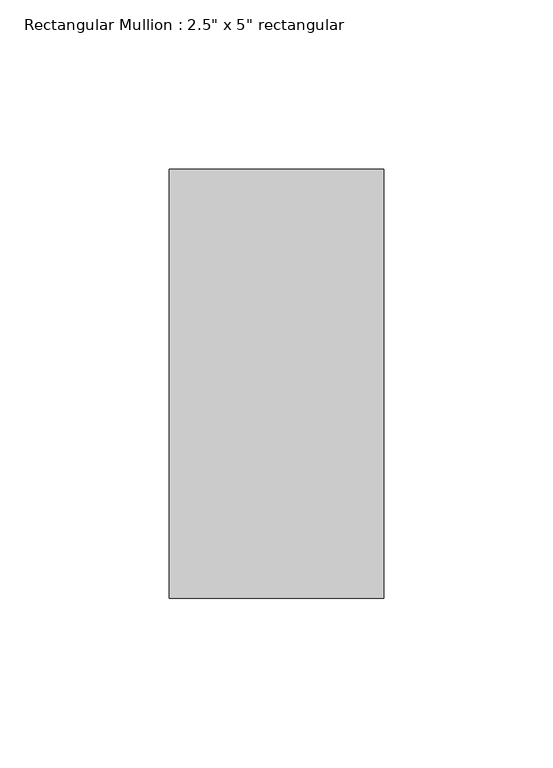
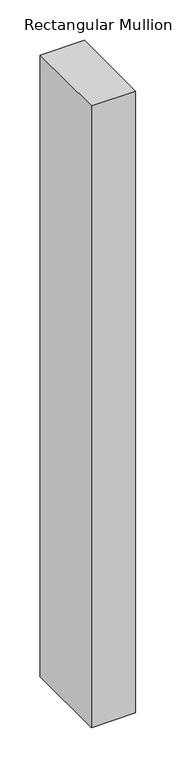
"""IFC4 building model written with IfcOpenShell, lengths in millimetres: member geometry."""

from ifc_helpers import new_model, si_unit, frame, origin, place, context, project, spatial, polyline, outline, extrude, source, transform, mapped, element, save


def member_f902c3b7(model_context):
    return source(origin(), model_context, "Body", "SweptSolid", [
        extrude(outline(polyline([(0.0, 63.5), (0.0, -63.5), (-63.5, -63.5), (-63.5, 63.5), (0.0, 63.5)])), frame((0.0, 0.0, -940.9162788), z_axis=(0.0, 0.0, 1.0), x_axis=(1.0, 0.0, 0.0)), (0.0, 0.0, 1.0), 940.9162788),
    ])


if __name__ == "__main__":
    model = new_model("IFC4")
    model_context = context("Model", 3, world=origin())
    ifc_project = project(units=[si_unit("LENGTHUNIT", "METRE", prefix="MILLI")], contexts=[model_context])
    site = spatial("IfcSite", under=ifc_project)
    building = spatial("IfcBuilding", under=site)
    placement = place(None, origin())
    member_shape = member_f902c3b7(model_context)
    element("IfcMember", 1, ObjectType="Rectangular Mullion : 2.5\" x 5\" rectangular", at=placement, inside=building, context=model_context, shape_type="MappedRepresentation", body=[
        mapped(member_shape, transform((0.0, 0.0, 0.0), x_axis=(1.0, 0.0, 0.0), y_axis=(0.0, 1.0, 0.0), z_axis=(0.0, 0.0, 1.0))),
    ])
    save(model, "model.ifc")

# Revit data of these elements
# Type "Rectangular Mullion : 2.5\" x 5\" rectangular"
#   built-in parameter 1007304 = 0.416667 (stored number, unit not read)
#   built-in parameter 1007301 = 0.104167 (stored number, unit not read)
#   built-in parameter 1007300 = 0.104167 (stored number, unit not read)
# Element 1 (IfcMember, "Rectangular Mullion : 2.5\" x 5\" rectangular")
#   Materials on its faces: "Aluminum"
# Materials
#   "Aluminum": class "Metal", colour RGB 247 247 247, transparency 0, Description = "Aluminum 6061", Cost = 0
